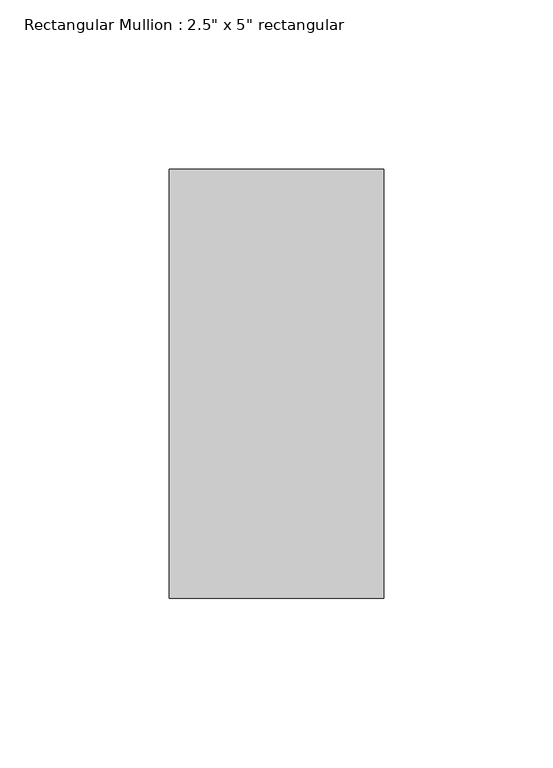
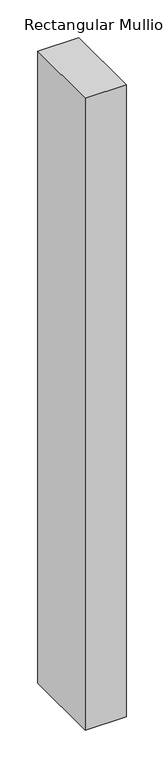
"""IFC4 building model written with IfcOpenShell, lengths in millimetres: member geometry."""

from ifc_helpers import new_model, si_unit, frame, origin, place, context, project, spatial, polyline, outline, extrude, source, transform, mapped, element, save


def member_456a42a1(model_context):
    return source(origin(), model_context, "Body", "SweptSolid", [
        extrude(outline(polyline([(0.0, 63.5), (0.0, -63.5), (-63.5, -63.5), (-63.5, 63.5), (0.0, 63.5)])), frame((0.0, 0.0, -1028.6999998), z_axis=(0.0, 0.0, 1.0), x_axis=(1.0, 0.0, 0.0)), (0.0, 0.0, 1.0), 1028.6999998),
    ])


if __name__ == "__main__":
    model = new_model("IFC4")
    model_context = context("Model", 3, world=origin())
    ifc_project = project(units=[si_unit("LENGTHUNIT", "METRE", prefix="MILLI")], contexts=[model_context])
    site = spatial("IfcSite", under=ifc_project)
    building = spatial("IfcBuilding", under=site)
    placement = place(None, origin())
    member_shape = member_456a42a1(model_context)
    element("IfcMember", 1, ObjectType="Rectangular Mullion : 2.5\" x 5\" rectangular", at=placement, inside=building, context=model_context, shape_type="MappedRepresentation", body=[
        mapped(member_shape, transform((0.0, 0.0, 0.0), x_axis=(1.0, 0.0, 0.0), y_axis=(0.0, 1.0, 0.0), z_axis=(0.0, 0.0, 1.0))),
    ])
    save(model, "model.ifc")

# Revit data of these elements
# Type "Rectangular Mullion : 2.5\" x 5\" rectangular"
#   built-in parameter 1007304 = 0.416667 (stored number, unit not read)
#   built-in parameter 1007301 = 0.104167 (stored number, unit not read)
#   built-in parameter 1007300 = 0.104167 (stored number, unit not read)
# Element 1 (IfcMember, "Rectangular Mullion : 2.5\" x 5\" rectangular")
#   Materials on its faces: "Aluminum"
# Materials
#   "Aluminum": class "Metal", colour RGB 247 247 247, transparency 0, Description = "Aluminum 6061", Cost = 0
